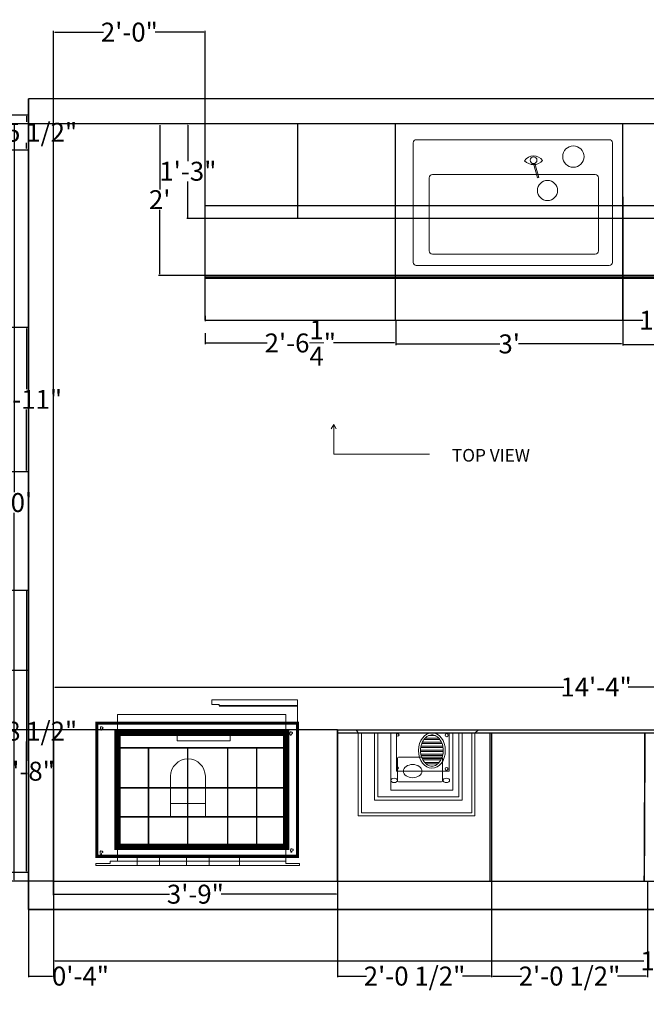
# Model space of a CAD drawing. Units: inches. Extents: x 1686244 to 1686928, y 1936095 to 1936489.
# Tile 10 of 11: x 1686702 to 1686801, y 1936330 to 1936486. Entities that reach past the tile are written whole.
import ezdxf

# ---------------------------------------------------------------- set-up
doc = ezdxf.new("R2010")
doc.units = ezdxf.units.IN
doc.header["$MEASUREMENT"] = 0
for name, color, linetype, lineweight in [('A-ANNO-DIMS', 240, 'Continuous', 18), ('A-ANNO-TEXT', 7, 'Continuous', 18), ('A-CASE', 7, 'Continuous', 35), ('A-ELEV', 7, 'Continuous', 25), ('A-ELEV-PATT', 72, 'Continuous', 13), ('A-FURN', 40, 'Continuous', 18)]:
    doc.layers.add(name, color=color, linetype=linetype, lineweight=lineweight)
doc.styles.get("Standard").update_dxf_attribs({"font": 'arial.ttf'})
doc.dimstyles.get("Standard").update_dxf_attribs({"dimtxt": 3, "dimasz": 0.18, "dimexe": 0.18, "dimexo": 0.0625, "dimgap": 0.09, "dimtad": 0, "dimtih": 1, "dimtoh": 1, "dimzin": 0, "dimdsep": 46, "dimlunit": 4, "dimtxsty": 'Standard', "dimcen": 0.09, "dimadec": 0, "dimazin": 0, "dimtfac": 1, "dimtofl": 0, "dimtmove": 0, "dimatfit": 3, "dimfxl": 1, "dimtolj": 1, "dimtzin": 0, "dimarcsym": 0})

# ---------------------------------------------------------------- blocks, each defined once
blk = doc.blocks.new('*D21')
at = {"layer": 'A-ANNO-DIMS', "color": 0, "lineweight": -2, "transparency": 16777216}
for p, q in [((1686707.33, 1936344.88), (1686707.33, 1936336.62)), ((1686904.33, 1936344.88), (1686904.33, 1936336.62)), ((1686707.51, 1936336.8), (1686800.91, 1936336.8)), ((1686904.15, 1936336.8), (1686811.11, 1936336.8))]:
    blk.add_line(p, q, dxfattribs=at)
at = {"layer": 'A-ANNO-DIMS', "color": 0, "transparency": 16777216}
for points in [[(1686707.51, 1936336.83), (1686707.51, 1936336.77), (1686707.33, 1936336.8)], [(1686904.15, 1936336.83), (1686904.15, 1936336.77), (1686904.33, 1936336.8)]]:
    blk.add_solid(points, dxfattribs=at)
at = {"layer": 'Defpoints', "color": 0, "transparency": 16777216}
for p in [(1686707.33, 1936344.94), (1686904.33, 1936344.94), (1686904.33, 1936336.8)]:
    blk.add_point(p, dxfattribs=at)
at = {"layer": 'A-ANNO-DIMS', "color": 0, "transparency": 16777216, "insert": (1686806.01, 1936336.8), "char_height": 3, "attachment_point": 5}
blk.add_mtext('\\A1;16\'-5"', dxfattribs=at)
blk = doc.blocks.new('*D26')
at = {"layer": 'A-ANNO-DIMS', "color": 0, "lineweight": -2, "transparency": 16777216}
for p, q in [((1686731.33, 1936439.01), (1686731.33, 1936438.16)), ((1686880.33, 1936439.01), (1686880.33, 1936438.16)), ((1686731.51, 1936438.34), (1686800.73, 1936438.34)), ((1686880.15, 1936438.34), (1686810.93, 1936438.34))]:
    blk.add_line(p, q, dxfattribs=at)
at = {"layer": 'A-ANNO-DIMS', "color": 0, "transparency": 16777216}
for points in [[(1686731.51, 1936438.37), (1686731.51, 1936438.31), (1686731.33, 1936438.34)], [(1686880.15, 1936438.37), (1686880.15, 1936438.31), (1686880.33, 1936438.34)]]:
    blk.add_solid(points, dxfattribs=at)
at = {"layer": 'Defpoints', "color": 0, "transparency": 16777216}
for p in [(1686731.33, 1936439.07), (1686880.33, 1936439.07), (1686731.33, 1936438.34)]:
    blk.add_point(p, dxfattribs=at)
at = {"layer": 'A-ANNO-DIMS', "color": 0, "transparency": 16777216, "insert": (1686805.83, 1936438.34), "char_height": 3, "attachment_point": 5}
blk.add_mtext('\\A1;12\'-5"', dxfattribs=at)
blk = doc.blocks.new('*D27')
at = {"layer": 'A-ANNO-DIMS', "color": 0, "lineweight": -2, "transparency": 16777216}
for p, q in [((1686761.56, 1936438.28), (1686761.56, 1936434.55)), ((1686731.33, 1936436.28), (1686731.33, 1936434.55)), ((1686731.51, 1936434.73), (1686741.2, 1936434.73)), ((1686761.38, 1936434.73), (1686751.68, 1936434.73))]:
    blk.add_line(p, q, dxfattribs=at)
at = {"layer": 'A-ANNO-DIMS', "color": 0, "transparency": 16777216}
for points in [[(1686731.51, 1936434.76), (1686731.51, 1936434.7), (1686731.33, 1936434.73)], [(1686761.38, 1936434.76), (1686761.38, 1936434.7), (1686761.56, 1936434.73)]]:
    blk.add_solid(points, dxfattribs=at)
at = {"layer": 'Defpoints', "color": 0, "transparency": 16777216}
for p in [(1686761.56, 1936438.34), (1686731.33, 1936436.34), (1686761.56, 1936434.73)]:
    blk.add_point(p, dxfattribs=at)
at = {"layer": 'A-ANNO-DIMS', "color": 0, "transparency": 16777216, "insert": (1686746.44, 1936434.73), "char_height": 3, "attachment_point": 5}
blk.add_mtext('\\A1;2\'-6{\\H1x;\\S1/4;}"', dxfattribs=at)
blk = doc.blocks.new('*D28')
at = {"layer": 'A-ANNO-DIMS', "color": 0, "lineweight": -2, "transparency": 16777216}
for p, q in [((1686761.56, 1936438.28), (1686761.56, 1936434.4)), ((1686797.56, 1936438.28), (1686797.56, 1936434.4)), ((1686761.74, 1936434.58), (1686778.09, 1936434.58)), ((1686797.38, 1936434.58), (1686781.03, 1936434.58))]:
    blk.add_line(p, q, dxfattribs=at)
at = {"layer": 'A-ANNO-DIMS', "color": 0, "transparency": 16777216}
for points in [[(1686761.74, 1936434.61), (1686761.74, 1936434.55), (1686761.56, 1936434.58)], [(1686797.38, 1936434.61), (1686797.38, 1936434.55), (1686797.56, 1936434.58)]]:
    blk.add_solid(points, dxfattribs=at)
at = {"layer": 'Defpoints', "color": 0, "transparency": 16777216}
for p in [(1686761.56, 1936438.34), (1686797.56, 1936438.34), (1686797.56, 1936434.58)]:
    blk.add_point(p, dxfattribs=at)
at = {"layer": 'A-ANNO-DIMS', "color": 0, "transparency": 16777216, "insert": (1686779.56, 1936434.58), "char_height": 3, "attachment_point": 5}
blk.add_mtext("\\A1;3'", dxfattribs=at)
blk = doc.blocks.new('*D29')
at = {"layer": 'A-ANNO-DIMS', "color": 0, "lineweight": -2, "transparency": 16777216}
for p, q in [((1686797.56, 1936438.28), (1686797.56, 1936434.32)), ((1686826.56, 1936438.28), (1686826.56, 1936434.32)), ((1686797.74, 1936434.5), (1686808.44, 1936434.5)), ((1686826.38, 1936434.5), (1686816.65, 1936434.5))]:
    blk.add_line(p, q, dxfattribs=at)
at = {"layer": 'A-ANNO-DIMS', "color": 0, "transparency": 16777216}
for points in [[(1686797.74, 1936434.53), (1686797.74, 1936434.47), (1686797.56, 1936434.5)], [(1686826.38, 1936434.53), (1686826.38, 1936434.47), (1686826.56, 1936434.5)]]:
    blk.add_solid(points, dxfattribs=at)
at = {"layer": 'Defpoints', "color": 0, "transparency": 16777216}
for p in [(1686797.56, 1936438.34), (1686826.56, 1936438.34), (1686826.56, 1936434.5)]:
    blk.add_point(p, dxfattribs=at)
at = {"layer": 'A-ANNO-DIMS', "color": 0, "transparency": 16777216, "insert": (1686812.54, 1936434.5), "char_height": 3, "attachment_point": 5}
blk.add_mtext('\\A1;2\'-5"', dxfattribs=at)
blk = doc.blocks.new('*D33')
at = {"layer": 'A-ANNO-DIMS', "color": 0, "lineweight": -2, "transparency": 16777216}
for p, q in [((1686731.26, 1936469.44), (1686728.43, 1936469.44)), ((1686728.61, 1936469.26), (1686728.61, 1936463.56)), ((1686728.61, 1936454.62), (1686728.61, 1936460.32)), ((1686731.26, 1936454.44), (1686728.43, 1936454.44))]:
    blk.add_line(p, q, dxfattribs=at)
at = {"layer": 'A-ANNO-DIMS', "color": 0, "transparency": 16777216}
for points in [[(1686728.58, 1936469.26), (1686728.64, 1936469.26), (1686728.61, 1936469.44)], [(1686728.58, 1936454.62), (1686728.64, 1936454.62), (1686728.61, 1936454.44)]]:
    blk.add_solid(points, dxfattribs=at)
at = {"layer": 'Defpoints', "color": 0, "transparency": 16777216}
for p in [(1686728.61, 1936469.44), (1686731.33, 1936469.44), (1686731.33, 1936454.44)]:
    blk.add_point(p, dxfattribs=at)
at = {"layer": 'A-ANNO-DIMS', "color": 0, "transparency": 16777216, "insert": (1686728.61, 1936461.94), "char_height": 3, "attachment_point": 5}
blk.add_mtext('\\A1;1\'-3"', dxfattribs=at)
blk = doc.blocks.new('*D34')
at = {"layer": 'A-ANNO-DIMS', "color": 0, "lineweight": -2, "transparency": 16777216}
for p, q in [((1686731.26, 1936469.44), (1686723.96, 1936469.44)), ((1686724.14, 1936469.26), (1686724.14, 1936459.04)), ((1686724.14, 1936445.62), (1686724.14, 1936455.85)), ((1686731.26, 1936445.44), (1686723.96, 1936445.44))]:
    blk.add_line(p, q, dxfattribs=at)
at = {"layer": 'A-ANNO-DIMS', "color": 0, "transparency": 16777216}
for points in [[(1686724.11, 1936469.26), (1686724.17, 1936469.26), (1686724.14, 1936469.44)], [(1686724.11, 1936445.62), (1686724.17, 1936445.62), (1686724.14, 1936445.44)]]:
    blk.add_solid(points, dxfattribs=at)
at = {"layer": 'Defpoints', "color": 0, "transparency": 16777216}
for p in [(1686724.14, 1936469.44), (1686731.33, 1936469.44), (1686731.33, 1936445.44)]:
    blk.add_point(p, dxfattribs=at)
at = {"layer": 'A-ANNO-DIMS', "color": 0, "transparency": 16777216, "insert": (1686724.14, 1936457.44), "char_height": 3, "attachment_point": 5}
blk.add_mtext("\\A1;2'", dxfattribs=at)
blk = doc.blocks.new('*D35')
at = {"layer": 'A-ANNO-DIMS', "color": 0, "lineweight": -2, "transparency": 16777216}
for p, q in [((1686707.33, 1936377.76), (1686707.33, 1936380.38)), ((1686707.51, 1936380.2), (1686788.23, 1936380.2)), ((1686879.15, 1936380.2), (1686798.43, 1936380.2)), ((1686879.33, 1936377.76), (1686879.33, 1936380.38))]:
    blk.add_line(p, q, dxfattribs=at)
at = {"layer": 'A-ANNO-DIMS', "color": 0, "transparency": 16777216}
for points in [[(1686707.51, 1936380.23), (1686707.51, 1936380.17), (1686707.33, 1936380.2)], [(1686879.15, 1936380.23), (1686879.15, 1936380.17), (1686879.33, 1936380.2)]]:
    blk.add_solid(points, dxfattribs=at)
at = {"layer": 'Defpoints', "color": 0, "transparency": 16777216}
for p in [(1686879.33, 1936380.2), (1686707.33, 1936377.7), (1686879.33, 1936377.7)]:
    blk.add_point(p, dxfattribs=at)
at = {"layer": 'A-ANNO-DIMS', "color": 0, "transparency": 16777216, "insert": (1686793.33, 1936380.2), "char_height": 3, "attachment_point": 5}
blk.add_mtext('\\A1;14\'-4"', dxfattribs=at)
blk = doc.blocks.new('*D36')
at = {"layer": 'A-ANNO-DIMS', "color": 0, "lineweight": -2, "transparency": 16777216}
for p, q in [((1686707.26, 1936469.44), (1686700.9, 1936469.44)), ((1686701.08, 1936469.26), (1686701.08, 1936411.06)), ((1686701.08, 1936349.62), (1686701.08, 1936407.82)), ((1686707.26, 1936349.44), (1686700.9, 1936349.44))]:
    blk.add_line(p, q, dxfattribs=at)
at = {"layer": 'A-ANNO-DIMS', "color": 0, "transparency": 16777216}
for points in [[(1686701.05, 1936469.26), (1686701.11, 1936469.26), (1686701.08, 1936469.44)], [(1686701.05, 1936349.62), (1686701.11, 1936349.62), (1686701.08, 1936349.44)]]:
    blk.add_solid(points, dxfattribs=at)
at = {"layer": 'Defpoints', "color": 0, "transparency": 16777216}
for p in [(1686707.33, 1936469.44), (1686701.08, 1936349.44), (1686707.33, 1936349.44)]:
    blk.add_point(p, dxfattribs=at)
at = {"layer": 'A-ANNO-DIMS', "color": 0, "transparency": 16777216, "insert": (1686701.08, 1936409.44), "char_height": 3, "attachment_point": 5}
blk.add_mtext("\\A1;10'", dxfattribs=at)
blk = doc.blocks.new('*D63')
at = {"layer": 'A-ANNO-DIMS', "color": 0, "lineweight": -2, "transparency": 16777216}
for p, q in [((1686707.26, 1936349.38), (1686707.26, 1936347.19)), ((1686752.33, 1936349.38), (1686752.33, 1936347.19)), ((1686707.44, 1936347.37), (1686725.72, 1936347.37)), ((1686752.15, 1936347.37), (1686733.87, 1936347.37))]:
    blk.add_line(p, q, dxfattribs=at)
at = {"layer": 'A-ANNO-DIMS', "color": 0, "transparency": 16777216}
for points in [[(1686707.44, 1936347.4), (1686707.44, 1936347.34), (1686707.26, 1936347.37)], [(1686752.15, 1936347.4), (1686752.15, 1936347.34), (1686752.33, 1936347.37)]]:
    blk.add_solid(points, dxfattribs=at)
at = {"layer": 'Defpoints', "color": 0, "transparency": 16777216}
for p in [(1686707.26, 1936349.44), (1686752.33, 1936349.44), (1686752.33, 1936347.37)]:
    blk.add_point(p, dxfattribs=at)
at = {"layer": 'A-ANNO-DIMS', "color": 0, "transparency": 16777216, "insert": (1686729.8, 1936347.37), "char_height": 3, "attachment_point": 5}
blk.add_mtext('\\A1;3\'-9"', dxfattribs=at)
blk = doc.blocks.new('*D102')
at = {"layer": 'A-ANNO-DIMS', "color": 0, "lineweight": -2, "transparency": 16777216}
for p, q in [((1686687.32, 1936395.55), (1686703.19, 1936395.55)), ((1686703.01, 1936395.37), (1686703.01, 1936374.85)), ((1686703.01, 1936351.04), (1686703.01, 1936371.57)), ((1686687.32, 1936350.86), (1686703.19, 1936350.86))]:
    blk.add_line(p, q, dxfattribs=at)
at = {"layer": 'A-ANNO-DIMS', "color": 0, "transparency": 16777216}
for points in [[(1686702.98, 1936395.37), (1686703.04, 1936395.37), (1686703.01, 1936395.55)], [(1686702.98, 1936351.04), (1686703.04, 1936351.04), (1686703.01, 1936350.86)]]:
    blk.add_solid(points, dxfattribs=at)
at = {"layer": 'Defpoints', "color": 0, "transparency": 16777216}
for p in [(1686687.26, 1936395.55), (1686687.26, 1936350.86), (1686703.01, 1936350.86)]:
    blk.add_point(p, dxfattribs=at)
at = {"layer": 'A-ANNO-DIMS', "color": 0, "transparency": 16777216, "insert": (1686703.01, 1936373.21), "char_height": 3, "attachment_point": 5}
blk.add_mtext('\\A1;3\'-8 1/2"', dxfattribs=at)
blk = doc.blocks.new('*D103')
at = {"layer": 'A-ANNO-DIMS', "color": 0, "lineweight": -2, "transparency": 16777216}
for p, q in [((1686687.32, 1936382.86), (1686703.19, 1936382.86)), ((1686703.01, 1936382.68), (1686703.01, 1936368.49)), ((1686703.01, 1936351.04), (1686703.01, 1936365.24)), ((1686687.32, 1936350.86), (1686703.19, 1936350.86))]:
    blk.add_line(p, q, dxfattribs=at)
at = {"layer": 'A-ANNO-DIMS', "color": 0, "transparency": 16777216}
for points in [[(1686702.98, 1936382.68), (1686703.04, 1936382.68), (1686703.01, 1936382.86)], [(1686702.98, 1936351.04), (1686703.04, 1936351.04), (1686703.01, 1936350.86)]]:
    blk.add_solid(points, dxfattribs=at)
at = {"layer": 'Defpoints', "color": 0, "transparency": 16777216}
for p in [(1686687.26, 1936382.86), (1686687.26, 1936350.86), (1686703.01, 1936350.86)]:
    blk.add_point(p, dxfattribs=at)
at = {"layer": 'A-ANNO-DIMS', "color": 0, "transparency": 16777216, "insert": (1686703.01, 1936366.86), "char_height": 3, "attachment_point": 5}
blk.add_mtext('\\A1;2\'-8"', dxfattribs=at)
blk = doc.blocks.new('*D104')
at = {"layer": 'A-ANNO-DIMS', "color": 0, "lineweight": -2, "transparency": 16777216}
for p, q in [((1686687.32, 1936470.86), (1686703.19, 1936470.86)), ((1686703.01, 1936470.68), (1686703.01, 1936469.75)), ((1686703.01, 1936465.54), (1686703.01, 1936466.47)), ((1686687.32, 1936465.36), (1686703.19, 1936465.36))]:
    blk.add_line(p, q, dxfattribs=at)
at = {"layer": 'A-ANNO-DIMS', "color": 0, "transparency": 16777216}
for points in [[(1686702.98, 1936470.68), (1686703.04, 1936470.68), (1686703.01, 1936470.86)], [(1686702.98, 1936465.54), (1686703.04, 1936465.54), (1686703.01, 1936465.36)]]:
    blk.add_solid(points, dxfattribs=at)
at = {"layer": 'Defpoints', "color": 0, "transparency": 16777216}
for p in [(1686687.26, 1936470.86), (1686687.26, 1936465.36), (1686703.01, 1936465.36)]:
    blk.add_point(p, dxfattribs=at)
at = {"layer": 'A-ANNO-DIMS', "color": 0, "transparency": 16777216, "insert": (1686703.01, 1936468.11), "char_height": 3, "attachment_point": 5}
blk.add_mtext('\\A1;0\'-5 1/2"', dxfattribs=at)
blk = doc.blocks.new('*D105')
at = {"layer": 'A-ANNO-DIMS', "color": 0, "lineweight": -2, "transparency": 16777216}
for p, q in [((1686634.84, 1936437.21), (1686703.19, 1936437.21)), ((1686703.01, 1936437.03), (1686703.01, 1936427.38)), ((1686703.01, 1936414.54), (1686703.01, 1936424.19)), ((1686634.82, 1936414.36), (1686703.19, 1936414.36))]:
    blk.add_line(p, q, dxfattribs=at)
at = {"layer": 'A-ANNO-DIMS', "color": 0, "transparency": 16777216}
for points in [[(1686702.98, 1936437.03), (1686703.04, 1936437.03), (1686703.01, 1936437.21)], [(1686702.98, 1936414.54), (1686703.04, 1936414.54), (1686703.01, 1936414.36)]]:
    blk.add_solid(points, dxfattribs=at)
at = {"layer": 'Defpoints', "color": 0, "transparency": 16777216}
for p in [(1686634.78, 1936437.21), (1686634.76, 1936414.36), (1686703.01, 1936414.36)]:
    blk.add_point(p, dxfattribs=at)
at = {"layer": 'A-ANNO-DIMS', "color": 0, "transparency": 16777216, "insert": (1686703.01, 1936425.79), "char_height": 3, "attachment_point": 5}
blk.add_mtext('\\A1;1\'-11"', dxfattribs=at)
blk = doc.blocks.new('*D106')
at = {"layer": 'A-ANNO-DIMS', "color": 0, "lineweight": -2, "transparency": 16777216}
for p, q in [((1686707.33, 1936349.38), (1686707.33, 1936334.21)), ((1686703.33, 1936344.88), (1686703.33, 1936334.21)), ((1686703.51, 1936334.39), (1686707.15, 1936334.39)), ((1686707.33, 1936334.39), (1686707.51, 1936334.39))]:
    blk.add_line(p, q, dxfattribs=at)
at = {"layer": 'A-ANNO-DIMS', "color": 0, "transparency": 16777216}
for points in [[(1686703.51, 1936334.42), (1686703.51, 1936334.36), (1686703.33, 1936334.39)], [(1686707.15, 1936334.42), (1686707.15, 1936334.36), (1686707.33, 1936334.39)]]:
    blk.add_solid(points, dxfattribs=at)
at = {"layer": 'Defpoints', "color": 0, "transparency": 16777216}
for p in [(1686707.33, 1936349.44), (1686703.33, 1936344.94), (1686707.33, 1936334.39)]:
    blk.add_point(p, dxfattribs=at)
at = {"layer": 'A-ANNO-DIMS', "color": 0, "transparency": 16777216, "insert": (1686711.58, 1936334.39), "char_height": 3, "attachment_point": 5}
blk.add_mtext('\\A1;0\'-4"', dxfattribs=at)
blk = doc.blocks.new('*D107')
at = {"layer": 'A-ANNO-DIMS', "color": 0, "lineweight": -2, "transparency": 16777216}
for p, q in [((1686752.33, 1936349.38), (1686752.33, 1936334.21)), ((1686776.77, 1936349.38), (1686776.77, 1936334.21)), ((1686752.51, 1936334.39), (1686756.95, 1936334.39)), ((1686776.59, 1936334.39), (1686772.15, 1936334.39))]:
    blk.add_line(p, q, dxfattribs=at)
at = {"layer": 'A-ANNO-DIMS', "color": 0, "transparency": 16777216}
for points in [[(1686752.51, 1936334.42), (1686752.51, 1936334.36), (1686752.33, 1936334.39)], [(1686776.59, 1936334.42), (1686776.59, 1936334.36), (1686776.77, 1936334.39)]]:
    blk.add_solid(points, dxfattribs=at)
at = {"layer": 'Defpoints', "color": 0, "transparency": 16777216}
for p in [(1686752.33, 1936349.44), (1686776.77, 1936349.44), (1686776.77, 1936334.39)]:
    blk.add_point(p, dxfattribs=at)
at = {"layer": 'A-ANNO-DIMS', "color": 0, "transparency": 16777216, "insert": (1686764.55, 1936334.39), "char_height": 3, "attachment_point": 5}
blk.add_mtext('\\A1;2\'-0 1/2"', dxfattribs=at)
blk = doc.blocks.new('*D108')
at = {"layer": 'A-ANNO-DIMS', "color": 0, "lineweight": -2, "transparency": 16777216}
for p, q in [((1686776.77, 1936349.38), (1686776.77, 1936334.21)), ((1686801.47, 1936349.38), (1686801.47, 1936334.21)), ((1686776.95, 1936334.39), (1686781.52, 1936334.39)), ((1686801.29, 1936334.39), (1686796.72, 1936334.39))]:
    blk.add_line(p, q, dxfattribs=at)
at = {"layer": 'A-ANNO-DIMS', "color": 0, "transparency": 16777216}
for points in [[(1686776.95, 1936334.42), (1686776.95, 1936334.36), (1686776.77, 1936334.39)], [(1686801.29, 1936334.42), (1686801.29, 1936334.36), (1686801.47, 1936334.39)]]:
    blk.add_solid(points, dxfattribs=at)
at = {"layer": 'Defpoints', "color": 0, "transparency": 16777216}
for p in [(1686776.77, 1936349.44), (1686801.47, 1936349.44), (1686801.47, 1936334.39)]:
    blk.add_point(p, dxfattribs=at)
at = {"layer": 'A-ANNO-DIMS', "color": 0, "transparency": 16777216, "insert": (1686789.12, 1936334.39), "char_height": 3, "attachment_point": 5}
blk.add_mtext('\\A1;2\'-0 1/2"', dxfattribs=at)
blk = doc.blocks.new('*D110')
at = {"layer": 'A-ANNO-DIMS', "color": 0, "lineweight": -2, "transparency": 16777216}
for p, q in [((1686707.33, 1936469.5), (1686707.33, 1936484.17)), ((1686707.51, 1936483.99), (1686715.22, 1936483.99)), ((1686731.15, 1936483.99), (1686723.43, 1936483.99)), ((1686731.33, 1936469.5), (1686731.33, 1936484.17))]:
    blk.add_line(p, q, dxfattribs=at)
at = {"layer": 'A-ANNO-DIMS', "color": 0, "transparency": 16777216}
for points in [[(1686707.51, 1936484.02), (1686707.51, 1936483.96), (1686707.33, 1936483.99)], [(1686731.15, 1936484.02), (1686731.15, 1936483.96), (1686731.33, 1936483.99)]]:
    blk.add_solid(points, dxfattribs=at)
at = {"layer": 'Defpoints', "color": 0, "transparency": 16777216}
for p in [(1686731.33, 1936483.99), (1686707.33, 1936469.44), (1686731.33, 1936469.44)]:
    blk.add_point(p, dxfattribs=at)
at = {"layer": 'A-ANNO-DIMS', "color": 0, "transparency": 16777216, "insert": (1686719.33, 1936483.99), "char_height": 3, "attachment_point": 5}
blk.add_mtext('\\A1;2\'-0"', dxfattribs=at)
blk = doc.blocks.new('*D111')
at = {"layer": 'A-ANNO-DIMS', "color": 0, "lineweight": -2, "transparency": 16777216}
for p, q in [((1686707.26, 1936373.44), (1686692.6, 1936373.44)), ((1686692.78, 1936373.26), (1686692.78, 1936363.06)), ((1686692.78, 1936349.62), (1686692.78, 1936359.82)), ((1686707.26, 1936349.44), (1686692.6, 1936349.44))]:
    blk.add_line(p, q, dxfattribs=at)
at = {"layer": 'A-ANNO-DIMS', "color": 0, "transparency": 16777216}
for points in [[(1686692.75, 1936373.26), (1686692.81, 1936373.26), (1686692.78, 1936373.44)], [(1686692.75, 1936349.62), (1686692.81, 1936349.62), (1686692.78, 1936349.44)]]:
    blk.add_solid(points, dxfattribs=at)
at = {"layer": 'Defpoints', "color": 0, "transparency": 16777216}
for p in [(1686692.78, 1936373.44), (1686707.33, 1936373.44), (1686707.33, 1936349.44)]:
    blk.add_point(p, dxfattribs=at)
at = {"layer": 'A-ANNO-DIMS', "color": 0, "transparency": 16777216, "insert": (1686692.78, 1936361.44), "char_height": 3, "attachment_point": 5}
blk.add_mtext('\\A1;2\'-0"', dxfattribs=at)

msp = doc.modelspace()

# ---------------------------------------------------------------- hatches: boundary and pattern name
at = {"layer": 'A-ELEV-PATT'}
h = msp.add_hatch(dxfattribs=at)
h.set_pattern_fill('ANSI32', color=256, scale=1.697052, angle=135)
h.set_pattern_definition([(180, (585748.9159, 672467.6728), (-1e-16, -0.63639444972), []), (180, (585748.7038, 672467.8849), (-1e-16, -0.63639444972), [])])
edge = h.paths.add_edge_path()
edge.add_spline(control_points=[(1686769.101, 1936370.139), (1686769.101, 1936370.371), (1686769.077, 1936370.602), (1686768.954, 1936371.187), (1686768.816, 1936371.523), (1686768.453, 1936372.074), (1686768.229, 1936372.288), (1686767.752, 1936372.562), (1686767.499, 1936372.625), (1686766.998, 1936372.604), (1686766.747, 1936372.52), (1686766.28, 1936372.202), (1686766.065, 1936371.967), (1686765.728, 1936371.383), (1686765.606, 1936371.034), (1686765.488, 1936370.297), (1686765.492, 1936369.909), (1686765.625, 1936369.176), (1686765.755, 1936368.833), (1686766.104, 1936368.263), (1686766.323, 1936368.037), (1686766.795, 1936367.739), (1686767.046, 1936367.664), (1686767.547, 1936367.661), (1686767.799, 1936367.733), (1686768.272, 1936368.027), (1686768.492, 1936368.25), (1686768.844, 1936368.816), (1686768.975, 1936369.158), (1686769.082, 1936369.724), (1686769.101, 1936369.932), (1686769.101, 1936370.139)], knot_values=[-1.5707963, -1.5707963, -1.5707963, -1.5707963, -1.2989292, -1.2989292, -0.8552596, -0.8552596, -0.4115901, -0.4115901, 0.0320795, 0.0320795, 0.475749, 0.475749, 0.9194185, 0.9194185, 1.3630881, 1.3630881, 1.8067576, 1.8067576, 2.2504272, 2.2504272, 2.6940967, 2.6940967, 3.1377662, 3.1377662, 3.5814358, 3.5814358, 4.0251053, 4.0251053, 4.4687749, 4.4687749, 4.712389, 4.712389, 4.712389, 4.712389], degree=3, periodic=0)

# ---------------------------------------------------------------- linework, layer by layer
at = {"layer": 'A-ANNO-DIMS'}
for p, q in [((1686751.309, 1936421.104), (1686751.734, 1936421.814)), ((1686751.734, 1936421.814), (1686751.734, 1936417.09)), ((1686751.734, 1936421.814), (1686752.117, 1936421.104)), ((1686751.734, 1936417.09), (1686766.917, 1936417.09))]:
    msp.add_line(p, q, dxfattribs=at)
at = {"layer": 'A-CASE'}
for q in [(1686703.327, 1936473.442), (1686908.327, 1936344.942)]:
    msp.add_line((1686703.327, 1936344.942), q, dxfattribs=at)
at = {"layer": 'A-ELEV'}
for p, q in [((1686908.327, 1936473.442), (1686703.327, 1936473.442)), ((1686707.327, 1936349.442), (1686707.327, 1936469.442)), ((1686903.827, 1936469.442), (1686707.327, 1936469.442)), ((1686731.327, 1936438.341), (1686731.327, 1936469.442)), ((1686746.054, 1936454.442), (1686746.054, 1936469.442)), ((1686761.556, 1936438.341), (1686761.556, 1936469.442)), ((1686797.556, 1936438.341), (1686797.556, 1936469.442)), ((1686797.556, 1936457.879), (1686797.556, 1936438.341)), ((1686904.327, 1936456.442), (1686731.327, 1936456.442)), ((1686904.327, 1936454.442), (1686731.327, 1936454.442)), ((1686880.327, 1936445.442), (1686731.327, 1936445.442)), ((1686879.827, 1936445.342), (1686731.327, 1936445.342)), ((1686879.577, 1936445.097), (1686731.327, 1936445.097)), ((1686879.327, 1936444.942), (1686731.327, 1936444.942)), ((1686752.327, 1936373.442), (1686823.58, 1936373.442)), ((1686752.327, 1936373.442), (1686752.327, 1936349.442)), ((1686752.327, 1936372.942), (1686880.327, 1936372.942)), ((1686776.524, 1936349.442), (1686776.524, 1936372.942)), ((1686752.327, 1936349.442), (1686776.524, 1936349.442)), ((1686776.524, 1936349.442), (1686800.721, 1936349.442)), ((1686800.704, 1936349.442), (1686904.327, 1936349.442))]:
    msp.add_line(p, q, dxfattribs=at)
msp.add_lwpolyline([(1686707.327, 1936373.442), (1686707.327, 1936349.442), (1686752.327, 1936349.442), (1686752.327, 1936373.442), (1686707.327, 1936373.442)], dxfattribs=at)
at = {"layer": 'A-ELEV', "const_width": 0.25}
for points in [[(1686776.774, 1936349.442), (1686776.774, 1936372.942)], [(1686801.08, 1936372.942), (1686800.973, 1936349.442)]]:
    msp.add_lwpolyline(points, dxfattribs=at)
at = {"layer": 'A-FURN'}
for p, q in [((1686745.997, 1936378.157), (1686732.389, 1936378.157)), ((1686732.389, 1936378.157), (1686732.389, 1936377.458)), ((1686745.997, 1936374.461), (1686745.997, 1936378.157)), ((1686732.389, 1936377.458), (1686733.557, 1936377.458)), ((1686733.557, 1936377.458), (1686733.557, 1936377.238)), ((1686755.318, 1936373.442), (1686755.616, 1936372.942)), ((1686774.119, 1936372.942), (1686774.168, 1936372.942)), ((1686774.168, 1936372.942), (1686774.694, 1936373.442)), ((1686725.87, 1936359.63), (1686725.87, 1936366.049)), ((1686731.38, 1936366.049), (1686731.38, 1936359.63)), ((1686725.87, 1936361.768), (1686731.38, 1936361.768)), ((1686714.012, 1936352.246), (1686716.291, 1936352.246)), ((1686716.291, 1936352.246), (1686716.291, 1936352.59)), ((1686744.12, 1936352.246), (1686744.12, 1936352.59)), ((1686746.324, 1936352.246), (1686744.12, 1936352.246))]:
    msp.add_line(p, q, dxfattribs=at)
for points in [[(1686764.831, 1936466.945), (1686795.426, 1936466.945, -0.4142136), (1686795.926, 1936466.445), (1686795.926, 1936447.495, -0.4142136), (1686795.426, 1936446.995), (1686764.831, 1936446.995, -0.4142136), (1686764.331, 1936447.495), (1686764.331, 1936466.445, -0.4142136)], [(1686767.388, 1936461.421), (1686793.198, 1936461.421, -0.4142136), (1686793.698, 1936460.921), (1686793.698, 1936449.308, -0.4142136), (1686793.198, 1936448.808), (1686767.388, 1936448.808, -0.4142136), (1686766.888, 1936449.308), (1686766.888, 1936460.921, -0.4142136)], [(1686762.099, 1936369.087), (1686768.753, 1936369.087, -0.4142136), (1686769.003, 1936368.837), (1686769.003, 1936365.406, -0.4142136), (1686768.753, 1936365.156), (1686762.099, 1936365.156, -0.4142136), (1686761.849, 1936365.406), (1686761.849, 1936368.837, -0.4142136)]]:
    msp.add_lwpolyline(points, format="xyb", close=True, dxfattribs=at)
for points in [[(1686783.413, 1936463.147), (1686783.625, 1936463.19), (1686784.256, 1936460.955), (1686784.051, 1936460.897)], [(1686717.459, 1936375.839), (1686744.13, 1936375.839), (1686744.13, 1936352.59), (1686717.459, 1936352.59)], [(1686726.908, 1936372.942), (1686735.321, 1936372.942), (1686735.321, 1936371.655), (1686726.908, 1936371.655)], [(1686761.669, 1936372.942), (1686770.035, 1936372.942), (1686770.035, 1936366.872), (1686761.669, 1936366.872)]]:
    msp.add_lwpolyline(points, close=True, dxfattribs=at)
at = {"layer": 'A-FURN', "const_width": 0.25}
for points in [[(1686733.557, 1936377.238), (1686745.997, 1936377.238)], [(1686717.459, 1936370.56), (1686744.13, 1936370.56)], [(1686722.382, 1936370.56), (1686722.382, 1936354.864)], [(1686728.584, 1936370.56), (1686728.584, 1936354.859)], [(1686734.92, 1936370.56), (1686734.92, 1936354.864)], [(1686739.522, 1936370.56), (1686739.522, 1936354.864)], [(1686717.459, 1936364.215), (1686744.197, 1936364.215)], [(1686717.459, 1936359.63), (1686744.197, 1936359.63)]]:
    msp.add_lwpolyline(points, dxfattribs=at)
at = {"layer": 'A-FURN'}
for points, const_width in [([(1686714.162, 1936374.461), (1686745.997, 1936374.461), (1686745.997, 1936353.364), (1686714.162, 1936353.364)], 0.5), ([(1686717.459, 1936372.942), (1686744.197, 1936372.942), (1686744.197, 1936354.864), (1686717.459, 1936354.864)], 1)]:
    msp.add_lwpolyline(points, close=True, dxfattribs=dict(at, const_width=const_width))
for points in [[(1686774.119, 1936372.942), (1686774.119, 1936359.771), (1686755.616, 1936359.771), (1686755.616, 1936372.942)], [(1686773.619, 1936372.942), (1686773.619, 1936360.271), (1686756.116, 1936360.271), (1686756.116, 1936372.942)], [(1686772.084, 1936372.942), (1686772.084, 1936362.288), (1686758.22, 1936362.288), (1686758.22, 1936372.942)], [(1686771.584, 1936372.942), (1686771.584, 1936362.788), (1686758.72, 1936362.788), (1686758.72, 1936372.942)], [(1686770.629, 1936372.942), (1686770.629, 1936363.876), (1686760.765, 1936363.876), (1686760.765, 1936372.942)], [(1686720.594, 1936353.364), (1686720.594, 1936351.901)], [(1686724.108, 1936353.311), (1686724.108, 1936351.901)], [(1686728.386, 1936353.364), (1686728.386, 1936351.901)], [(1686731.997, 1936353.364), (1686731.997, 1936351.901)], [(1686736.821, 1936353.364), (1686736.821, 1936351.901)], [(1686746.324, 1936352.246), (1686746.324, 1936351.901), (1686714.012, 1936351.901), (1686714.012, 1936352.246)], [(1686716.291, 1936352.59), (1686744.13, 1936352.59)]]:
    msp.add_lwpolyline(points, dxfattribs=at)
for centre, radius in [((1686789.731, 1936464.272), 1.693), ((1686783.413, 1936463.693), 0.546), ((1686785.635, 1936458.888), 1.6), ((1686761.898, 1936372.606), 0.189), ((1686769.651, 1936372.576), 0.248), ((1686761.849, 1936367.381), 0.174), ((1686769.632, 1936367.23), 0.238)]:
    msp.add_circle(centre, radius, dxfattribs=at)
for centre, radius, start, end in [((1686783.436, 1936462.608), 1.756, 36.15161, 145.34955), ((1686783.405, 1936464.913), 1.925, 222.73014, 318.77101), ((1686728.625, 1936366.049), 2.755, 0, 180)]:
    msp.add_arc(centre, radius, start, end, dxfattribs=at)
for centre, major_axis, ratio in [((1686767.303, 1936370.139), (0, 2.803), 0.7579577), ((1686764.256, 1936366.872), (1.476, 0), 0.710716)]:
    msp.add_ellipse(centre, major_axis=major_axis, ratio=ratio, start_param=-1.5707963, end_param=4.712389, dxfattribs=at)
for centre in [(1686761.324, 1936365.406), (1686769.591, 1936365.396)]:
    msp.add_ellipse(centre, major_axis=(-0.525, 0), ratio=0.6503015, dxfattribs=at)
for points, knots in [([(1686714.786, 1936373.39), (1686714.767, 1936373.464), (1686714.735, 1936373.587), (1686714.764, 1936373.742), (1686714.775, 1936373.982), (1686715.166, 1936373.884), (1686715.175, 1936373.585), (1686714.875, 1936373.6), (1686714.97, 1936373.345), (1686714.851, 1936373.374), (1686714.786, 1936373.39)], [0, 0, 0, 0, 0.2229476, 0.3728812, 0.4860538, 0.8632462, 0.9781918, 1.2435366, 1.3678283, 1.5125124, 1.5125124, 1.5125124, 1.5125124]), ([(1686744.826, 1936372.573), (1686744.807, 1936372.647), (1686744.775, 1936372.77), (1686744.804, 1936372.926), (1686744.815, 1936373.166), (1686745.206, 1936373.067), (1686745.215, 1936372.769), (1686744.915, 1936372.784), (1686745.01, 1936372.528), (1686744.89, 1936372.558), (1686744.826, 1936372.573)], [0, 0, 0, 0, 0.2229476, 0.3728812, 0.4860538, 0.8632462, 0.9781918, 1.2435366, 1.3678283, 1.5125124, 1.5125124, 1.5125124, 1.5125124]), ([(1686769.101, 1936370.139), (1686769.101, 1936370.371), (1686769.077, 1936370.602), (1686768.954, 1936371.187), (1686768.816, 1936371.523), (1686768.453, 1936372.074), (1686768.229, 1936372.288), (1686767.752, 1936372.562), (1686767.499, 1936372.625), (1686766.998, 1936372.604), (1686766.747, 1936372.52), (1686766.28, 1936372.202), (1686766.065, 1936371.967), (1686765.728, 1936371.383), (1686765.606, 1936371.034), (1686765.488, 1936370.297), (1686765.492, 1936369.909), (1686765.625, 1936369.176), (1686765.755, 1936368.833), (1686766.104, 1936368.263), (1686766.323, 1936368.037), (1686766.795, 1936367.739), (1686767.046, 1936367.664), (1686767.547, 1936367.661), (1686767.799, 1936367.733), (1686768.272, 1936368.027), (1686768.492, 1936368.25), (1686768.844, 1936368.816), (1686768.975, 1936369.158), (1686769.082, 1936369.724), (1686769.101, 1936369.932), (1686769.101, 1936370.139)], [-1.5707963, -1.5707963, -1.5707963, -1.5707963, -1.2989292, -1.2989292, -0.8552596, -0.8552596, -0.4115901, -0.4115901, 0.0320795, 0.0320795, 0.475749, 0.475749, 0.9194185, 0.9194185, 1.3630881, 1.3630881, 1.8067576, 1.8067576, 2.2504272, 2.2504272, 2.6940967, 2.6940967, 3.1377662, 3.1377662, 3.5814358, 3.5814358, 4.0251053, 4.0251053, 4.4687749, 4.4687749, 4.712389, 4.712389, 4.712389, 4.712389]), ([(1686714.747, 1936353.697), (1686714.728, 1936353.771), (1686714.696, 1936353.894), (1686714.725, 1936354.049), (1686714.736, 1936354.289), (1686715.127, 1936354.191), (1686715.136, 1936353.892), (1686714.836, 1936353.907), (1686714.931, 1936353.652), (1686714.811, 1936353.681), (1686714.747, 1936353.697)], [0, 0, 0, 0, 0.2229476, 0.3728812, 0.4860538, 0.8632462, 0.9781918, 1.2435366, 1.3678283, 1.5125124, 1.5125124, 1.5125124, 1.5125124]), ([(1686744.936, 1936354.048), (1686744.917, 1936354.122), (1686744.885, 1936354.245), (1686744.914, 1936354.401), (1686744.925, 1936354.641), (1686745.316, 1936354.542), (1686745.325, 1936354.244), (1686745.025, 1936354.259), (1686745.12, 1936354.003), (1686745, 1936354.033), (1686744.936, 1936354.048)], [0, 0, 0, 0, 0.2229476, 0.3728812, 0.4860538, 0.8632462, 0.9781918, 1.2435366, 1.3678283, 1.5125124, 1.5125124, 1.5125124, 1.5125124])]:
    msp.add_open_spline(points, degree=3, knots=knots, dxfattribs=at)

# ---------------------------------------------------------------- texts
at = {"layer": 'A-ANNO-TEXT'}
msp.add_text('TOP VIEW', height=2, dxfattribs=at).set_placement((1686770.481, 1936415.924))

# ---------------------------------------------------------------- dimensions: what is measured, and where the dimension line sits
at = {"layer": 'A-ANNO-DIMS'}
for base, p1, p2, override, picture, middle in [((1686731.327, 1936483.992), (1686707.327, 1936469.442), (1686731.327, 1936469.442), {"dimdec": 1, "dimlfac": 1, "dimrnd": 0, "dimzin": 1, "dimdsep": 46, "dimlunit": 4, "dimfrac": 2}, '*D110', (1686719.327, 1936483.992)), ((1686731.327, 1936438.341), (1686880.327, 1936439.075), (1686731.327, 1936439.075), {"dimclrd": 0, "dimclre": 0, "dimclrt": 0}, '*D26', (1686805.827, 1936438.341)), ((1686707.327, 1936334.392), (1686703.327, 1936344.942), (1686707.327, 1936349.442), {"dimdec": 1, "dimlfac": 1, "dimrnd": 0, "dimzin": 1, "dimdsep": 46, "dimlunit": 4, "dimfrac": 2}, '*D106', (1686711.585, 1936334.392)), ((1686752.327, 1936347.37), (1686707.265, 1936349.442), (1686752.327, 1936349.442), {"dimclrd": 0, "dimclre": 0, "dimclrt": 0}, '*D63', (1686729.796, 1936347.37)), ((1686776.774, 1936334.392), (1686752.327, 1936349.442), (1686776.774, 1936349.442), {"dimdec": 1, "dimlfac": 1, "dimrnd": 0, "dimzin": 1, "dimdsep": 46, "dimlunit": 4, "dimfrac": 2}, '*D107', (1686764.551, 1936334.392)), ((1686801.471, 1936334.392), (1686776.774, 1936349.442), (1686801.471, 1936349.442), {"dimdec": 1, "dimlfac": 1, "dimrnd": 0, "dimzin": 1, "dimdsep": 46, "dimlunit": 4, "dimfrac": 2}, '*D108', (1686789.123, 1936334.392))]:
    dim = msp.add_linear_dim(base=base, p1=p1, p2=p2, dimstyle='Standard', override=override, dxfattribs=at)
    dim.commit()
    dim.dimension.update_dxf_attribs({"geometry": picture, "text_midpoint": middle})
for base, p1, p2, override, picture, middle in [((1686703.009, 1936465.364), (1686687.259, 1936470.864), (1686687.259, 1936465.364), {"dimdec": 1, "dimlfac": 1, "dimrnd": 0, "dimzin": 1, "dimdsep": 46, "dimlunit": 4, "dimfrac": 2}, '*D104', (1686703.009, 1936468.114)), ((1686701.079, 1936349.442), (1686707.327, 1936469.442), (1686707.327, 1936349.442), {"dimclrd": 0, "dimclre": 0, "dimclrt": 0}, '*D36', (1686701.079, 1936409.442)), ((1686724.14, 1936469.442), (1686731.327, 1936445.442), (1686731.327, 1936469.442), {"dimclrd": 0, "dimclre": 0, "dimclrt": 0}, '*D34', (1686724.14, 1936457.442)), ((1686728.612, 1936469.442), (1686731.327, 1936454.442), (1686731.327, 1936469.442), {"dimclrd": 0, "dimclre": 0, "dimclrt": 0}, '*D33', (1686728.612, 1936461.942)), ((1686703.009, 1936414.364), (1686634.778, 1936437.211), (1686634.758, 1936414.364), {"dimdec": 1, "dimlfac": 1, "dimrnd": 0, "dimzin": 1, "dimdsep": 46, "dimlunit": 4, "dimfrac": 2}, '*D105', (1686703.009, 1936425.787)), ((1686703.009, 1936350.864), (1686687.259, 1936395.552), (1686687.259, 1936350.864), {"dimdec": 1, "dimlfac": 1, "dimrnd": 0, "dimzin": 1, "dimdsep": 46, "dimlunit": 4, "dimfrac": 2}, '*D102', (1686703.009, 1936373.208)), ((1686703.009, 1936350.864), (1686687.259, 1936382.864), (1686687.259, 1936350.864), {"dimdec": 1, "dimlfac": 1, "dimrnd": 0, "dimzin": 1, "dimdsep": 46, "dimlunit": 4, "dimfrac": 2}, '*D103', (1686703.009, 1936366.864)), ((1686692.777, 1936373.442), (1686707.327, 1936349.442), (1686707.327, 1936373.442), {"dimdec": 1, "dimlfac": 1, "dimrnd": 0, "dimzin": 1, "dimdsep": 46, "dimlunit": 4, "dimfrac": 2}, '*D111', (1686692.777, 1936361.442))]:
    dim = msp.add_linear_dim(base=base, p1=p1, p2=p2, angle=90, dimstyle='Standard', override=override, dxfattribs=at)
    dim.commit()
    dim.dimension.update_dxf_attribs({"geometry": picture, "text_midpoint": middle})
for base, p1, p2, picture, middle in [((1686761.556, 1936434.734), (1686731.327, 1936436.343), (1686761.556, 1936438.341), '*D27', (1686746.442, 1936434.734)), ((1686797.556, 1936434.583), (1686761.556, 1936438.341), (1686797.556, 1936438.341), '*D28', (1686779.556, 1936434.583)), ((1686826.556, 1936434.502), (1686797.556, 1936438.341), (1686826.556, 1936438.341), '*D29', (1686812.543, 1936434.502)), ((1686879.327, 1936380.203), (1686707.327, 1936377.699), (1686879.327, 1936377.699), '*D35', (1686793.327, 1936380.203)), ((1686904.327, 1936336.8), (1686707.327, 1936344.942), (1686904.327, 1936344.942), '*D21', (1686806.007, 1936336.8))]:
    dim = msp.add_linear_dim(base=base, p1=p1, p2=p2, dimstyle='Standard', override={"dimclrd": 0, "dimclre": 0, "dimclrt": 0}, dxfattribs=at)
    dim.commit()
    dim.dimension.update_dxf_attribs({"geometry": picture, "text_midpoint": middle, "dimtype": 160})

doc.saveas('drawing.dxf')
